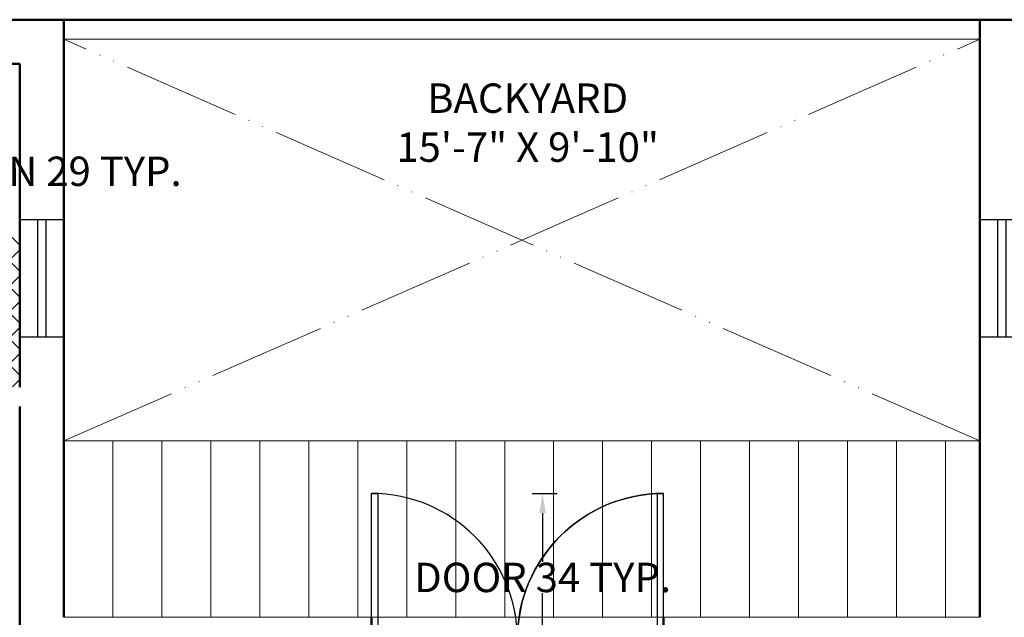
# Model space of a CAD drawing. Units: inches. Extents: x -466983 to 1020, y 324 to 318697.
# Tile 92 of 97: x 609 to 810, y 963 to 1085. Entities that reach past the tile are written whole.
import ezdxf

# ---------------------------------------------------------------- set-up
doc = ezdxf.new("R2010")
doc.units = ezdxf.units.IN
doc.header["$MEASUREMENT"] = 0
doc.linetypes.add('ACAD_ISO05W100', pattern=[33, 24, -3, 0, -3, 0, -3])
for name, color, linetype, lineweight in [('A-ANNO-DIMS', 2, 'Continuous', 18), ('A-ANNO-SYMB', 252, 'ACAD_ISO05W100', 18), ('A-AREA-IDEN', 7, 'Continuous', 25), ('A-DOOR', 3, 'Continuous', 25), ('A-FLOR-PATT', 252, 'Continuous', 13), ('A-GLAZ', 4, 'Continuous', 25), ('A-WALL', 7, 'Continuous', 50), ('L-SITE', 3, 'Continuous', 18)]:
    doc.layers.add(name, color=color, linetype=linetype, lineweight=lineweight)
doc.styles.get("Standard").update_dxf_attribs({"font": 'arial.ttf'})
doc.dimstyles.get("Standard").update_dxf_attribs({"dimtxt": 6, "dimasz": 4, "dimexe": 3, "dimexo": 3, "dimgap": 0.09, "dimtad": 0, "dimtih": 1, "dimtoh": 1, "dimdec": 1, "dimzin": 0, "dimdsep": 46, "dimlunit": 3, "dimtxsty": 'Standard', "dimcen": 0.09, "dimadec": 0, "dimazin": 0, "dimtfac": 1, "dimtdec": 1, "dimtofl": 0, "dimtmove": 0, "dimatfit": 3, "dimfxl": 1, "dimtolj": 1, "dimtzin": 0, "dimarcsym": 0})

# ---------------------------------------------------------------- blocks, each defined once
blk = doc.blocks.new('Ventilator')
for p, q in [((1433.59, 801.68), (1457.59, 801.68)), ((1433.59, 792.68), (1433.59, 801.68)), ((1457.59, 801.68), (1457.59, 792.68)), ((1433.59, 797.98), (1457.59, 797.98)), ((1457.59, 796.38), (1433.59, 796.38)), ((1457.59, 792.68), (1433.59, 792.68))]:
    blk.add_line(p, q)
blk = doc.blocks.new('*U39')
for p, q in [((0, 0), (0, -6)), ((-40, 0), (-40, -6))]:
    blk.add_line(p, q)
blk.add_lwpolyline([(0, 0), (0, 40), (-1.75, 40), (-1.75, 0)], close=True)
blk.add_arc((0, 0), 40, 90, 180)
blk = doc.blocks.new('*U41')
for p, q in [((0, 0), (0, -6)), ((40, 0), (40, -6))]:
    blk.add_line(p, q)
blk.add_lwpolyline([(0, 0), (0, 40), (1.75, 40), (1.75, 0)], close=True)
blk.add_arc((0, 0), 40, 0, 90)
blk = doc.blocks.new('DOOR-30IN')
for p, q in [((0, 4.47), (0, 0)), ((29.81, 4.47), (29.81, 0))]:
    blk.add_line(p, q)
blk.add_lwpolyline([(0, 4.47), (0, 34.28), (1.3, 34.28), (1.3, 4.47)], close=True)
blk.add_arc((0, 4.47), 29.81, 0, 90)
blk = doc.blocks.new('*D57')
at = {"layer": 'A-ANNO-DIMS', "color": 0, "lineweight": -2, "transparency": 16777216}
for p, q in [((713.4, 988.22), (718.55, 988.22)), ((715.55, 984.22), (715.55, 974.28)), ((715.55, 957.94), (715.55, 967.88)), ((713.4, 953.94), (718.55, 953.94))]:
    blk.add_line(p, q, dxfattribs=at)
at = {"layer": 'A-ANNO-DIMS', "color": 0, "transparency": 16777216}
for points in [[(714.88, 984.22), (716.21, 984.22), (715.55, 988.22)], [(714.88, 957.94), (716.21, 957.94), (715.55, 953.94)]]:
    blk.add_solid(points, dxfattribs=at)
at = {"layer": 'Defpoints', "color": 0, "transparency": 16777216}
for p in [(710.4, 988.22), (715.55, 988.22), (710.4, 953.94)]:
    blk.add_point(p, dxfattribs=at)
at = {"layer": 'A-ANNO-DIMS', "color": 0, "transparency": 16777216, "insert": (715.55, 971.08), "char_height": 6, "attachment_point": 5}
blk.add_mtext('\\A1;DOOR 34 TYP.', dxfattribs=at)
blk = doc.blocks.new('*D79')
at = {"layer": 'A-ANNO-DIMS', "color": 0, "lineweight": -2, "transparency": 16777216}
for p, q in [((529.67, 1055.35), (529.67, 1050.99)), ((558.73, 1055.35), (558.73, 1050.99)), ((533.67, 1053.99), (554.73, 1053.99)), ((558.73, 1053.99), (562.73, 1053.99))]:
    blk.add_line(p, q, dxfattribs=at)
at = {"layer": 'A-ANNO-DIMS', "color": 0, "transparency": 16777216}
for points in [[(533.67, 1054.66), (533.67, 1053.33), (529.67, 1053.99)], [(554.73, 1054.66), (554.73, 1053.33), (558.73, 1053.99)]]:
    blk.add_solid(points, dxfattribs=at)
at = {"layer": 'Defpoints', "color": 0, "transparency": 16777216}
for p in [(529.67, 1058.35), (558.73, 1058.35), (558.73, 1053.99)]:
    blk.add_point(p, dxfattribs=at)
at = {"layer": 'A-ANNO-DIMS', "color": 0, "transparency": 16777216, "insert": (603.86, 1053.99), "char_height": 6, "attachment_point": 5}
blk.add_mtext('\\A1;WASHBASIN 29 TYP.', dxfattribs=at)

msp = doc.modelspace()

# ---------------------------------------------------------------- hatches: boundary and pattern name
at = {"layer": 'A-FLOR-PATT', "transparency": 33554572}
h = msp.add_hatch(dxfattribs=at)
h.set_pattern_fill('ANSI37', color=256, scale=30)
h.set_pattern_definition([(45, (-1212.4137, -290.035), (-2.6516504, 2.6516504), []), (135, (-1212.4137, -290.035), (-2.6516504, -2.6516504), [])])
h.paths.add_polyline_path([(901.81, 1075.94), (900.61, 1075.94), (900.61, 1065.39), (899.39, 1065.39), (898.09, 1065.39), (892.84, 1058.71, -0.258377), (892.19, 1058.35), (879.98, 1058.35, -0.20177), (879.44, 1058.58), (874.08, 1065.39), (872.78, 1065.39), (871.56, 1065.39), (871.56, 1075.94), (813.81, 1075.94), (813.81, 1044.79), (832.39, 1044.79, -0.394795), (848.66, 1028.54), (848.66, 1009.94), (901.81, 1009.94), (901.81, 1015.94), (901.31, 1015.94), (871.31, 1015.94), (871.31, 1017.25), (871.33, 1017.25, -0.401453), (901.31, 1045.94), (901.81, 1045.94)])
edge = h.paths.add_edge_path(flags=16)
edge.add_line((847.77, 1068.95), (847.77, 1073.71))
edge.add_arc((849.23, 1073.71), 1.45, 90, 180, ccw=False)
edge.add_line((849.23, 1075.16), (864.49, 1075.16))
edge.add_arc((864.49, 1073.71), 1.45, 0, 90, ccw=False)
edge.add_line((865.95, 1073.71), (865.95, 1069))
edge.add_arc((832.64, 1068.98), 33.3, -20.6123, 0.0472, ccw=False)
edge.add_ellipse((856.86, 1058.48), major_axis=(0, 10.21), ratio=0.685919, start_angle=100.0088, end_angle=259.9912, ccw=False)
edge.add_arc((881.07, 1068.98), 33.3, 180.0472, 200.6123, ccw=False)
h.paths.add_polyline_path([(853.15, 1066.48), (853.15, 1066.45), (853.15, 1066.45, 0.433107), (852.92, 1066.68), (852.92, 1066.45), (853.15, 1066.45), (853.15, 1066.48), (853.09, 1066.61, 0.697939), (852.7, 1066.45), (852.7, 1066.45), (852.7, 1066.48), (852.92, 1067), (852.92, 1066.68, -0.396254)], flags=0)
h.paths.add_polyline_path([(861.02, 1066.48), (861.02, 1066.45), (861.02, 1066.45, 0.416404), (860.8, 1066.68), (860.8, 1066.45), (861.02, 1066.45), (861.02, 1066.48), (860.97, 1066.61, 0.713344), (860.57, 1066.45), (860.57, 1066.45), (860.57, 1066.48), (860.8, 1067), (860.8, 1066.68, -0.379973)], flags=0)
edge = h.paths.add_edge_path(flags=0)
edge.add_spline(control_points=[(861.13, 1065.79), (861.47, 1065.25), (861.61, 1065.02), (861.98, 1064.37), (862.19, 1063.94), (862.56, 1063.04), (862.72, 1062.56), (862.99, 1061.58), (863.09, 1061.07), (863.25, 1060.03), (863.29, 1059.5), (863.33, 1058.44), (863.32, 1057.91), (863.24, 1056.85), (863.17, 1056.33), (862.97, 1055.31), (862.84, 1054.81), (862.54, 1053.85), (862.36, 1053.39), (861.95, 1052.52), (861.73, 1052.12), (861.23, 1051.36), (860.97, 1051.02), (860.4, 1050.39), (860.11, 1050.12), (859.49, 1049.65), (859.18, 1049.45), (858.53, 1049.13), (858.2, 1049.01), (857.53, 1048.85), (857.2, 1048.81), (856.52, 1048.81), (856.19, 1048.85), (855.52, 1049.01), (855.19, 1049.13), (854.54, 1049.45), (854.23, 1049.64), (853.61, 1050.12), (853.32, 1050.39), (852.75, 1051.01), (852.49, 1051.36), (852, 1052.11), (851.77, 1052.52), (851.36, 1053.39), (851.18, 1053.85), (850.88, 1054.81), (850.75, 1055.31), (850.55, 1056.33), (850.48, 1056.85), (850.4, 1057.9), (850.39, 1058.44), (850.43, 1059.5), (850.47, 1060.03), (850.63, 1061.07), (850.73, 1061.58), (851, 1062.56), (851.16, 1063.04), (851.53, 1063.94), (851.73, 1064.37), (852.11, 1065.02), (852.25, 1065.25), (852.61, 1065.73)], knot_values=[3.915332, 3.915332, 3.915332, 3.915332, 4.013468, 4.013468, 4.175532, 4.175532, 4.337596, 4.337596, 4.49966, 4.49966, 4.661724, 4.661724, 4.823788, 4.823788, 4.985852, 4.985852, 5.147916, 5.147916, 5.30998, 5.30998, 5.472044, 5.472044, 5.634109, 5.634109, 5.796173, 5.796173, 5.958237, 5.958237, 6.120301, 6.120301, 6.282365, 6.282365, 6.444429, 6.444429, 6.606493, 6.606493, 6.768557, 6.768557, 6.930621, 6.930621, 7.092685, 7.092685, 7.254749, 7.254749, 7.416813, 7.416813, 7.578878, 7.578878, 7.740942, 7.740942, 7.903006, 7.903006, 8.06507, 8.06507, 8.227134, 8.227134, 8.389198, 8.389198, 8.551262, 8.551262, 8.65037, 8.65037, 8.65037, 8.65037], degree=3, periodic=0)
edge.add_line((852.64, 1065.79), (861.13, 1065.79))
edge = h.paths.add_edge_path(flags=0)
edge.add_ellipse((856.85, 1057.74), major_axis=(0, 7.79), ratio=0.687861, start_angle=0, end_angle=360)
h.paths.add_polyline_path([(848.86, 1069.39), (848.86, 1073.96, -0.414214), (849.95, 1075.05), (863.77, 1075.05, -0.414214), (864.86, 1073.96), (864.86, 1069.39, -0.388936), (864.52, 1069.03, -0.043561), (849.2, 1069.03, -0.388936)], flags=0)
h.paths.add_polyline_path([(853.1, 1068.11, -1), (852.68, 1068.11, -1)], flags=0)
edge = h.paths.add_edge_path(flags=0)
edge.add_ellipse((856.86, 1057.34), major_axis=(0, 2.21), ratio=0.657164, start_angle=0, end_angle=360)
h.paths.add_polyline_path([(861.04, 1068.11, -1), (860.62, 1068.11, -1)], flags=0)
edge = h.paths.add_edge_path()
edge.add_line((573.95, 1057.34), (573.95, 1075.94))
edge.add_line((573.95, 1075.94), (558.73, 1075.94))
edge.add_line((558.73, 1075.94), (558.73, 1065.39))
edge.add_line((558.73, 1065.39), (557.51, 1065.39))
edge.add_line((557.51, 1065.39), (556.21, 1065.39))
edge.add_line((556.21, 1065.39), (550.95, 1058.71))
edge.add_arc((550.3, 1059.12), 0.765, 270, 327.9483, ccw=False)
edge.add_line((550.3, 1058.35), (538.1, 1058.35))
edge.add_arc((538.1, 1059.12), 0.765, 224.3704, 270, ccw=False)
edge.add_line((537.55, 1058.58), (532.2, 1065.39))
edge.add_line((532.2, 1065.39), (530.9, 1065.39))
edge.add_line((530.9, 1065.39), (529.67, 1065.39))
edge.add_line((529.67, 1065.39), (529.67, 1075.94))
edge.add_line((529.67, 1075.94), (520.81, 1075.94))
edge.add_line((520.81, 1075.94), (520.81, 1045.94))
edge.add_line((520.81, 1045.94), (521.31, 1045.94))
edge.add_arc((521.31, 1015.94), 30, 2.5075, 90, ccw=False)
edge.add_line((551.28, 1017.25), (551.31, 1017.25))
edge.add_line((551.31, 1017.25), (551.31, 1015.94))
edge.add_line((551.31, 1015.94), (520.81, 1015.94))
edge.add_line((520.81, 1015.94), (520.81, 1009.94))
edge.add_line((520.81, 1009.94), (559.19, 1010.4))
edge.add_arc((559.19, 1011.86), 1.45, 180, 270, ccw=False)
edge.add_line((557.74, 1011.86), (557.74, 1016.56))
edge.add_arc((591.04, 1016.59), 33.3, 159.3877, 180.0472, ccw=False)
edge.add_ellipse((566.82, 1027.08), major_axis=(0, 10.21), ratio=0.685919, start_angle=280.0088, end_angle=439.9912, ccw=False)
edge.add_arc((542.61, 1016.59), 33.3, 0.0472, 20.6123, ccw=False)
edge.add_line((575.91, 1016.62), (575.91, 1011.86))
edge.add_arc((574.46, 1011.86), 1.45, -90, 0, ccw=False)
edge.add_line((574.46, 1010.4), (608.81, 1009.94))
edge.add_line((608.81, 1009.94), (608.81, 1041.09))
edge.add_line((608.81, 1041.09), (590.22, 1041.09))
edge.add_arc((590.78, 1057.91), 16.83, 181.9277, 268.1032, ccw=False)
edge = h.paths.add_edge_path()
edge.add_ellipse((494.24, 583.62), major_axis=(0, 10.21), ratio=0.685919, start_angle=280.0088, end_angle=439.9912, ccw=False)
edge.add_arc((470.03, 573.12), 33.3, 0.0472, 20.6123, ccw=False)
edge.add_line((503.33, 573.15), (503.33, 568.39))
edge.add_arc((501.88, 568.39), 1.45, -90, 0, ccw=False)
edge.add_line((501.88, 566.94), (539.81, 566.94))
edge.add_line((539.81, 566.94), (539.81, 572.94))
edge.add_line((539.81, 572.94), (539.31, 572.94))
edge.add_line((539.31, 572.94), (509.31, 572.94))
edge.add_line((509.31, 572.94), (509.31, 574.25))
edge.add_line((509.31, 574.25), (509.33, 574.25))
edge.add_arc((539.31, 572.94), 30, 90, 177.4925, ccw=False)
edge.add_line((539.31, 602.94), (539.81, 602.94))
edge.add_line((539.81, 602.94), (539.81, 626.94))
edge.add_line((539.81, 626.94), (531.77, 626.94))
edge.add_line((531.77, 626.94), (531.77, 616.39))
edge.add_line((531.77, 616.39), (530.55, 616.39))
edge.add_line((530.55, 616.39), (529.25, 616.39))
edge.add_line((529.25, 616.39), (523.71, 609.35))
edge.add_line((523.71, 609.35), (510.78, 609.35))
edge.add_line((510.78, 609.35), (505.24, 616.39))
edge.add_line((505.24, 616.39), (503.94, 616.39))
edge.add_line((503.94, 616.39), (502.72, 616.39))
edge.add_line((502.72, 616.39), (502.72, 626.94))
edge.add_line((502.72, 626.94), (481.7, 626.94))
edge.add_line((481.7, 626.94), (481.7, 611))
edge.add_arc((467.27, 611.47), 14.44, 271.9277, 358.1032, ccw=False)
edge.add_line((467.76, 597.05), (451.81, 597.05))
edge.add_line((451.81, 597.05), (451.81, 584.4))
edge.add_line((451.81, 584.4), (451.81, 566.94))
edge.add_line((451.81, 566.94), (486.61, 566.94))
edge.add_arc((486.61, 568.39), 1.45, 180, 270, ccw=False)
edge.add_line((485.16, 568.39), (485.16, 573.1))
edge.add_arc((518.46, 573.12), 33.3, 159.3877, 180.0472, ccw=False)
h.paths.add_polyline_path([(836.26, 1020.73), (879.89, 1020.73), (879.89, 1039.39), (836.26, 1039.39)], flags=25)
h.paths.add_polyline_path([(549.99, 1036.75), (593.61, 1036.75), (593.61, 1055.41), (549.99, 1055.41)], flags=24)
h.paths.add_polyline_path([(475.12, 595.6), (518.75, 595.6), (518.75, 614.25), (475.12, 614.25)], flags=24)

# ---------------------------------------------------------------- linework, layer by layer
at = {"layer": 'A-ANNO-SYMB'}
for p, q in [((617.81, 998.94), (804.81, 1080.94)), ((804.81, 998.94), (617.81, 1080.94))]:
    msp.add_line(p, q, dxfattribs=at)
at = {"layer": 'A-WALL'}
for p, q in [((391.81, 1084.94), (991.81, 1084.94)), ((617.81, 962.94), (617.81, 1084.94)), ((804.81, 1084.94), (804.81, 962.94)), ((520.81, 1075.94), (608.81, 1075.94)), ((608.81, 1009.94), (608.81, 1075.94)), ((608.81, 870.94), (608.81, 1005.94)), ((680.59, 962.94), (680.59, 953.94)), ((740.22, 962.94), (740.22, 953.94))]:
    msp.add_line(p, q, dxfattribs=at)
at = {"layer": 'L-SITE'}
for p, q in [((617.81, 1080.94), (804.81, 1080.94)), ((617.81, 998.94), (804.81, 998.94)), ((627.81, 962.94), (627.81, 998.94)), ((637.81, 962.94), (637.81, 998.94)), ((647.81, 962.94), (647.81, 998.94)), ((657.81, 962.94), (657.81, 998.94)), ((667.81, 962.94), (667.81, 998.94)), ((677.81, 962.94), (677.81, 998.94)), ((687.81, 962.94), (687.81, 998.94)), ((697.81, 962.94), (697.81, 998.94)), ((707.81, 962.94), (707.81, 998.94)), ((717.81, 962.94), (717.81, 998.94)), ((727.81, 962.94), (727.81, 998.94)), ((737.81, 962.94), (737.81, 998.94)), ((747.81, 962.94), (747.81, 998.94)), ((757.81, 962.94), (757.81, 998.94)), ((767.81, 962.94), (767.81, 998.94)), ((777.81, 962.94), (777.81, 998.94)), ((787.81, 962.94), (787.81, 998.94)), ((797.81, 962.94), (797.81, 998.94)), ((617.81, 962.94), (804.81, 962.94))]:
    msp.add_line(p, q, dxfattribs=at)

# ---------------------------------------------------------------- block references
at = {"layer": 'A-DOOR'}
for name, p, xscale, yscale, zscale in [('*U41', (680.59, 958.41), 0.7452984294347067, 0.7452984294347067, 0.7452984294347067), ('*U39', (740.22, 958.41), 0.7452984294346952, 0.7452984294346952, 0.7452984294346952)]:
    msp.add_blockref(name, p, dxfattribs=dict(at, xscale=xscale, yscale=yscale, zscale=zscale))
msp.add_blockref('DOOR-30IN', (680.59, 953.94), dxfattribs=at)
msp.add_blockref('DOOR-30IN', (680.59, 953.94), dxfattribs=at)
msp.add_blockref('DOOR-30IN', (680.59, 953.94), dxfattribs=at)
msp.add_blockref('DOOR-30IN', (680.59, 953.94), dxfattribs=at)
at = {"layer": 'A-DOOR', "extrusion": (0, 0, -1), "zscale": -1}
msp.add_blockref('DOOR-30IN', (-740.21, 953.94), dxfattribs=at)
msp.add_blockref('DOOR-30IN', (-740.21, 953.94), dxfattribs=at)
at = {"layer": 'A-GLAZ', "rotation": 270}
for p in [(-183.87, 2477.74), (12.13, 2477.74)]:
    msp.add_blockref('Ventilator', p, dxfattribs=at)

# ---------------------------------------------------------------- texts
at = {"layer": 'A-AREA-IDEN', "insert": (597.72, 1071.92), "char_height": 6, "attachment_point": 1}
msp.add_mtext_dynamic_manual_height_columns('\\pxqc;{\\fArial|b1|i0|c0|p34;BACKYARD\\P15\'-7" X 9\'-10"}', width=229.5583, gutter_width=1, heights=[0], dxfattribs=at)

# ---------------------------------------------------------------- dimensions: what is measured, and where the dimension line sits
at = {"layer": 'A-ANNO-DIMS'}
dim = msp.add_linear_dim(base=(558.73, 1053.99), p1=(529.67, 1058.35), p2=(558.73, 1058.35), text='WASHBASIN <> TYP.', dimstyle='Standard', override={"dimdec": 0, "dimlfac": 1, "dimrnd": 0, "dimzin": 0, "dimdsep": 46, "dimlunit": 2}, dxfattribs=at)
dim.commit()
dim.dimension.update_dxf_attribs({"geometry": '*D79', "text_midpoint": (603.86, 1053.99)})
dim = msp.add_linear_dim(base=(715.55, 988.22), p1=(710.4, 953.94), p2=(710.4, 988.22), angle=90, text='DOOR <> TYP.', dimstyle='Standard', override={"dimdec": 0, "dimlfac": 1, "dimrnd": 0, "dimzin": 0, "dimdsep": 46, "dimlunit": 2}, dxfattribs=at)
dim.commit()
dim.dimension.update_dxf_attribs({"geometry": '*D57', "text_midpoint": (715.55, 971.08)})

doc.saveas('drawing.dxf')
